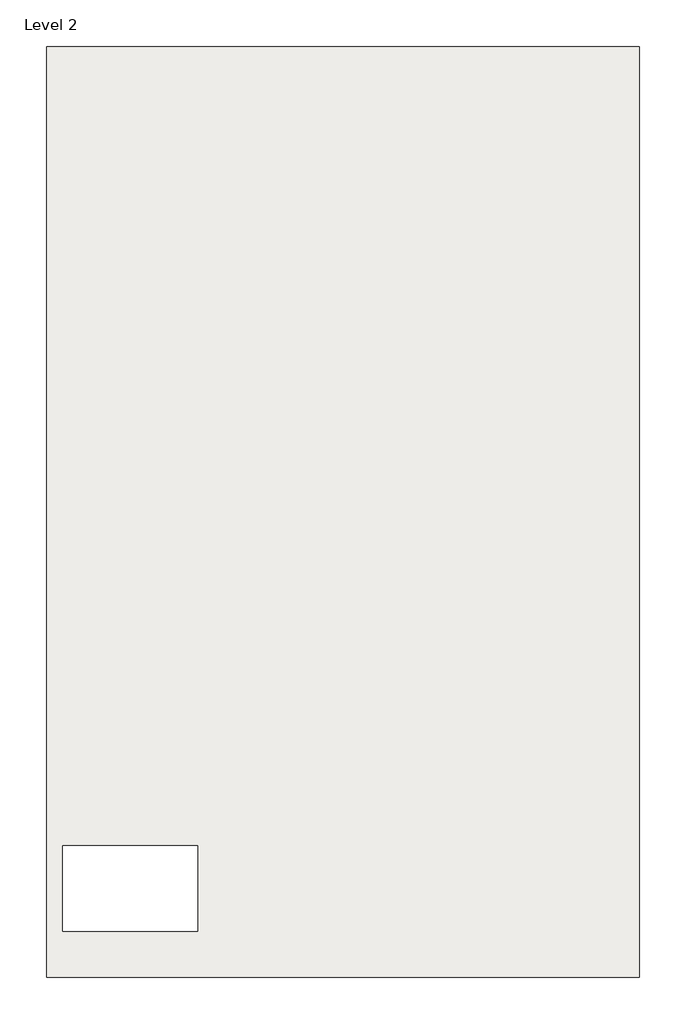
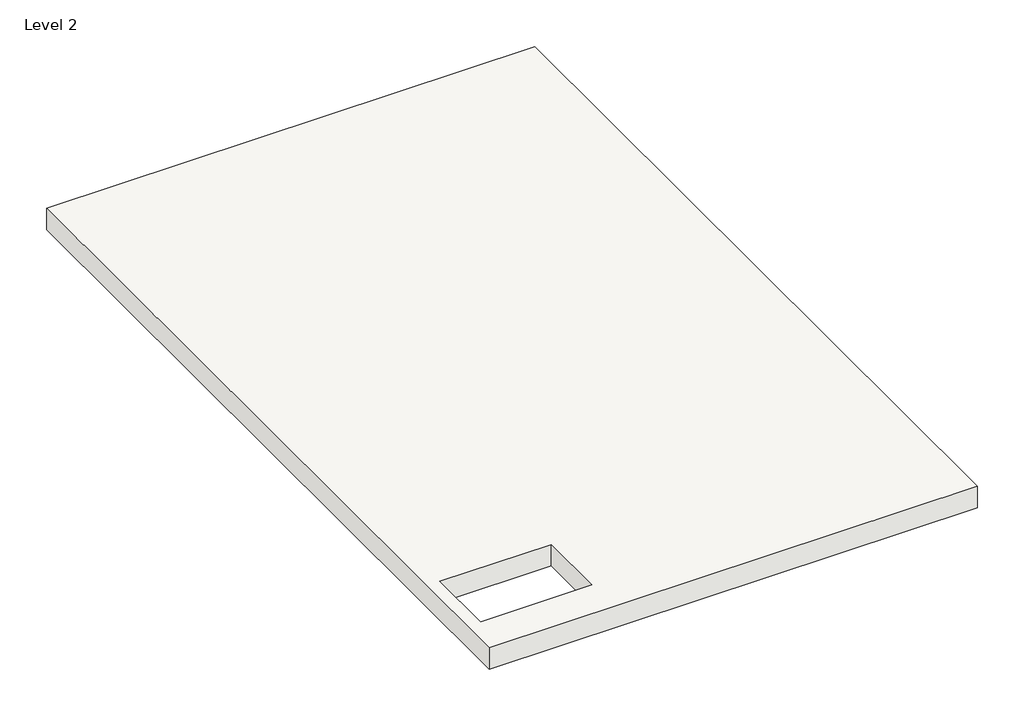
# One storey: 1 roof.
"""IFC4 building model written with IfcOpenShell, lengths in millimetres."""

from ifc_helpers import new_model, si_unit, frame, origin, place, context, project, spatial, polyline, outline, extrude, element, save

model = new_model("IFC4")

# Units and contexts
model_context = context("Model", 3, world=origin())
ifc_project = project(units=[si_unit("LENGTHUNIT", "METRE", prefix="MILLI")], contexts=[model_context])

# Site, building, storey
site = spatial("IfcSite", under=ifc_project)
building = spatial("IfcBuilding", under=site)
storey = spatial("IfcBuildingStorey", under=building, Name="Level 2", Elevation=3048.0)

# Roof
placement = place(None, origin())
element("IfcRoof", 1, ObjectType="Steel Truss - Insulation on Metal Deck - EPDM", at=placement, inside=storey, context=model_context, shape_type="SweptSolid", body=[
    extrude(outline(polyline([(-13649.931213, 14000.8633056), (-1838.931213, 14000.8633056), (-1838.931213, -4541.1366944), (-13649.931213, -4541.1366944), (-13649.931213, 14000.8633056)]), holes=[polyline([(-10636.560337, -3624.5366944), (-10636.560337, -1922.7366944), (-13328.960337, -1922.7366944), (-13328.960337, -3624.5366944), (-10636.560337, -3624.5366944)])]), frame((0.0, 0.0, 3048.0), z_axis=(0.0, 0.0, 1.0), x_axis=(1.0, 0.0, 0.0)), (0.0, 0.0, 1.0), 546.1),
])

save(model, "model.ifc")

# Revit data of these elements
# Type "Steel Truss - Insulation on Metal Deck - EPDM"
#   Assembly Code = "B1020"
#   Layers, outside or top first: 0' - 0 1/4" "Roofing, EPDM Membrane" (function 4); 0' - 5" "Rigid insulation" (function 3); 0' - 0 1/4" "Metal Deck" (function 1); 1' - 4" "Structure, Steel Bar Joist Layer" (function 1)
# Element 1 (IfcRoof, "Steel Truss - Insulation on Metal Deck - EPDM")
#   built-in parameter 1001705 = 11.7917 (stored number, unit not read)
#   built-in parameter 1001710 = 33615
#   Phase Created = New Construction
#   Materials on its faces: "Structure, Steel Bar Joist Layer", "Roofing, EPDM Membrane"
# Materials
#   "Roofing, EPDM Membrane": class "Generic", colour RGB 127 127 127, transparency 0, Description = "EPDM roof membrane", Cost = 0
#   "Rigid insulation": class "Generic", colour RGB 127 127 127, transparency 0, Description = "Rigid foam insulation board", Cost = 0
#   "Metal Deck": class "Metal", colour RGB 199 199 199, transparency 0, Description = "Steel, mill finish", Cost = 0
#   "Structure, Steel Bar Joist Layer": class "Metal", colour RGB 127 127 127, transparency 0, Description = "Bar joists, thermal airspace", Cost = 0
